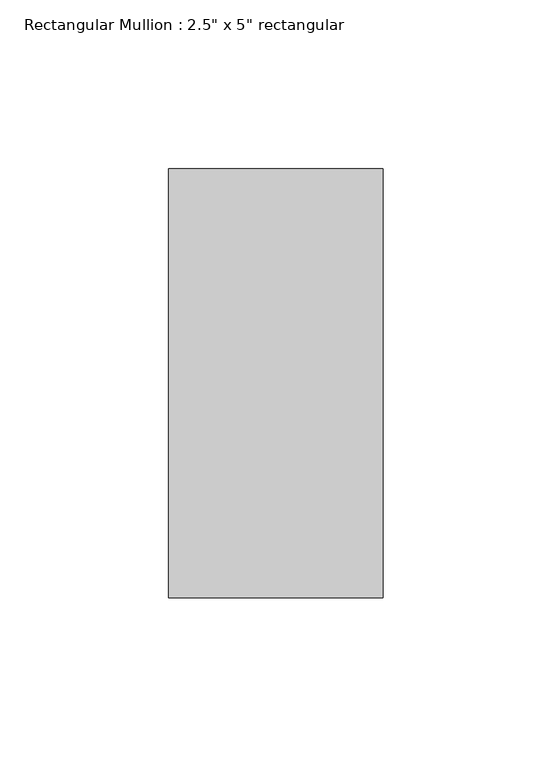
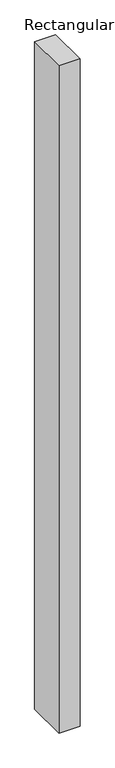
"""IFC4 building model written with IfcOpenShell, lengths in millimetres: member geometry."""

from ifc_helpers import new_model, si_unit, frame, origin, place, context, project, spatial, polyline, outline, extrude, source, transform, mapped, element, save


def member_3374d9b6(model_context):
    return source(origin(), model_context, "Body", "SweptSolid", [
        extrude(outline(polyline([(0.0, 63.5), (0.0, -63.5), (-63.5, -63.5), (-63.5, 63.5), (0.0, 63.5)])), frame((0.0, 0.0, -2133.6), z_axis=(0.0, 0.0, 1.0), x_axis=(1.0, 0.0, 0.0)), (0.0, 0.0, 1.0), 2133.6),
    ])


if __name__ == "__main__":
    model = new_model("IFC4")
    model_context = context("Model", 3, world=origin())
    ifc_project = project(units=[si_unit("LENGTHUNIT", "METRE", prefix="MILLI")], contexts=[model_context])
    site = spatial("IfcSite", under=ifc_project)
    building = spatial("IfcBuilding", under=site)
    placement = place(None, origin())
    member_shape = member_3374d9b6(model_context)
    element("IfcMember", 1, ObjectType="Rectangular Mullion : 2.5\" x 5\" rectangular", at=placement, inside=building, context=model_context, shape_type="MappedRepresentation", body=[
        mapped(member_shape, transform((0.0, 0.0, 0.0), x_axis=(1.0, 0.0, 0.0), y_axis=(0.0, 1.0, 0.0), z_axis=(0.0, 0.0, 1.0))),
    ])
    save(model, "model.ifc")

# Revit data of these elements
# Type "Rectangular Mullion : 2.5\" x 5\" rectangular"
#   built-in parameter 1007304 = 0.416667 (stored number, unit not read)
#   built-in parameter 1007301 = 0.104167 (stored number, unit not read)
#   built-in parameter 1007300 = 0.104167 (stored number, unit not read)
# Element 1 (IfcMember, "Rectangular Mullion : 2.5\" x 5\" rectangular")
#   Materials on its faces: "door black"
# Materials
#   "door black": class "Generic", colour RGB 120 120 120, transparency 0, Cost = 0
